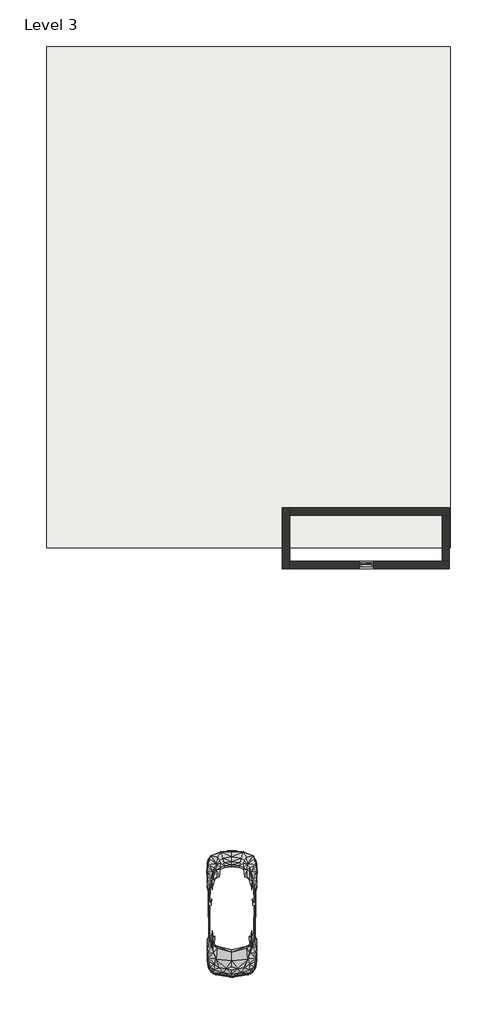
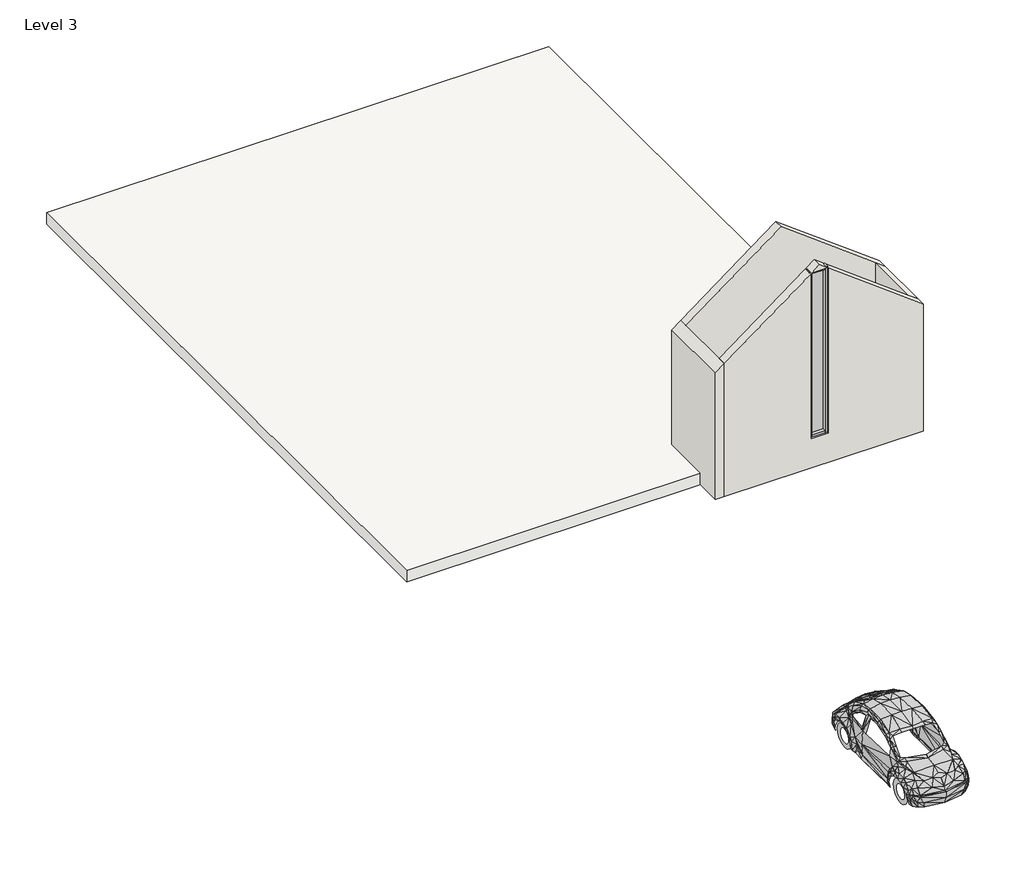
# One storey: 4 members, 4 walls, 1 plate, 1 proxy, 1 roof.
"""IFC4 building model written with IfcOpenShell, lengths in millimetres."""

from ifc_helpers import new_model, si_unit, frame, origin, place, context, project, spatial, polyline, outline, extrude, faceted_brep, transform, mapped, element, save
from components import rpc_beetle_rpc_beetle_31f8b51e, member_ff9f2d30, member_ad6a65ad, system_panel_glazed_5fe90612

model = new_model("IFC4")

# Units and contexts
model_context = context("Model", 3, world=origin())
ifc_project = project(units=[si_unit("LENGTHUNIT", "METRE", prefix="MILLI")], contexts=[model_context])

# Site, building, storey
site = spatial("IfcSite", under=ifc_project)
building = spatial("IfcBuilding", under=site)
storey = spatial("IfcBuildingStorey", under=building, Name="Level 3", Elevation=6096.0)

# Proxy
placement = place(None, origin())
rpc_beetle_rpc_beetle_shape = rpc_beetle_rpc_beetle_31f8b51e(model_context)
element("IfcBuildingElementProxy", 1, Name="RPC Beetle : RPC Beetle", ObjectType="RPC Beetle : RPC Beetle", at=placement, inside=storey, context=model_context, shape_type="MappedRepresentation", body=[
    mapped(rpc_beetle_rpc_beetle_shape, transform((-17655.2886697, -22453.5511954, 6096.0), x_axis=(-1.0, 0.0, 0.0), y_axis=(0.0, -1.0, 0.0), z_axis=(0.0, 0.0, 1.0))),
])

# Members
member_shape = member_ff9f2d30(model_context)
element("IfcMember", 2, ObjectType="Rectangular Mullion : 2.5\" x 5\" rectangular", at=placement, inside=storey, context=model_context, shape_type="MappedRepresentation", body=[
    mapped(member_shape, transform((-13610.3386697, -12750.7511954, 6863.106036), x_axis=(0.0, 0.0, -1.0), y_axis=(0.0, -1.0, 0.0), z_axis=(-1.0, 0.0, 0.0))),
])
element("IfcMember", 3, ObjectType="Rectangular Mullion : 2.5\" x 5\" rectangular", at=placement, inside=storey, context=model_context, shape_type="MappedRepresentation", body=[
    mapped(member_shape, transform((-13280.1386697, -12750.7511954, 11278.5636215), x_axis=(0.0, 0.0, 1.0), y_axis=(0.0, -1.0, 0.0), z_axis=(1.0, 0.0, 0.0))),
])
member_2_shape = member_ad6a65ad(model_context)
element("IfcMember", 4, ObjectType="Rectangular Mullion : 2.5\" x 5\" rectangular", at=placement, inside=storey, context=model_context, shape_type="MappedRepresentation", body=[
    mapped(member_2_shape, transform((-13673.8386697, -12750.7511954, 11278.5636215), x_axis=(-1.0, 0.0, 0.0), y_axis=(0.0, -1.0, 0.0), z_axis=(0.0, 0.0, 1.0))),
])
element("IfcMember", 5, ObjectType="Rectangular Mullion : 2.5\" x 5\" rectangular", at=placement, inside=storey, context=model_context, shape_type="MappedRepresentation", body=[
    mapped(member_2_shape, transform((-13216.6386697, -12750.7511954, 6863.106036), x_axis=(1.0, 0.0, 0.0), y_axis=(0.0, -1.0, 0.0), z_axis=(0.0, 0.0, -1.0))),
])

# Plate
system_panel_glazed_shape = system_panel_glazed_5fe90612(model_context)
element("IfcPlate", 6, ObjectType="System Panel : Glazed", at=placement, inside=storey, context=model_context, shape_type="MappedRepresentation", body=[
    mapped(system_panel_glazed_shape, transform((-13445.2386697, -12750.7511954, 6926.606036), x_axis=(1.0, 0.0, 0.0), y_axis=(0.0, 1.0, 0.0), z_axis=(0.0, 0.0, 1.0))),
])

# Roof
element("IfcRoof", 7, ObjectType="Generic - 12\"", at=placement, inside=storey, context=model_context, shape_type="SweptSolid", body=[
    extrude(outline(polyline([(-23465.5386697, 3492.5488046), (-10816.3386697, 3492.5488046), (-10816.3386697, -12204.6511954), (-23465.5386697, -12204.6511954), (-23465.5386697, 3492.5488046)])), frame((0.0, 0.0, 6096.0), z_axis=(0.0, 0.0, 1.0), x_axis=(1.0, 0.0, 0.0)), (0.0, 0.0, 1.0), 304.8),
])

# Walls
element("IfcWall", 8, ObjectType="9\"", at=placement, inside=storey, context=model_context, shape_type="Brep", body=[
    faceted_brep([(-15845.5386697, -12865.0511954, 6096.0), (-15845.5386697, -12636.4511954, 6096.0), (-15845.5386697, -11191.8261954, 6096.0), (-15845.5386697, -10963.2261954, 6096.0), (-15845.5386697, -10963.2261954, 9631.8623433), (-15845.5386697, -11191.8261954, 9631.8623433), (-15845.5386697, -12636.4511954, 9631.8623433), (-15845.5386697, -12865.0511954, 9631.8623433), (-16074.1386697, -12865.0511954, 6096.0), (-16074.1386697, -12865.0511954, 9460.4123433), (-16074.1386697, -10963.2261954, 9460.4123433), (-16074.1386697, -10963.2261954, 6096.0)], [[[0, 1, 2, 3, 4, 5, 6, 7]], [[8, 9, 10, 11]], [[3, 2, 1, 0, 8, 11]], [[4, 3, 11, 10]], [[0, 7, 9, 8]], [[7, 6, 5, 4, 10, 9]]]),
])
element("IfcWall", 9, ObjectType="9\"", at=placement, inside=storey, context=model_context, shape_type="Brep", body=[
    faceted_brep([(-15845.5386697, -11191.8261954, 6096.0), (-11070.3386697, -11191.8261954, 6096.0), (-10841.7386697, -11191.8261954, 6096.0), (-10841.7386697, -11191.8261954, 9471.8166443), (-11070.3386697, -11191.8261954, 9643.2666443), (-13450.3358024, -11191.8261954, 11428.2644938), (-15845.5386697, -11191.8261954, 9631.8623433), (-15845.5386697, -10963.2261954, 6096.0), (-15845.5386697, -10963.2261954, 9631.8623433), (-13450.3358024, -10963.2261954, 11428.2644938), (-10841.7386697, -10963.2261954, 9471.8166443), (-10841.7386697, -10963.2261954, 6096.0)], [[[0, 1, 2, 3, 4, 5, 6]], [[7, 8, 9, 10, 11]], [[2, 1, 0, 7, 11]], [[0, 6, 8, 7]], [[3, 2, 11, 10]], [[6, 5, 9, 8]], [[5, 4, 3, 10, 9]]]),
])
element("IfcWall", 10, ObjectType="9\"", at=placement, inside=storey, context=model_context, shape_type="Brep", body=[
    faceted_brep([(-15845.5386697, -12865.0511954, 6096.0), (-10841.7386697, -12865.0511954, 6096.0), (-10841.7386697, -12865.0511954, 9471.8166443), (-13216.6386697, -12865.0511954, 11252.9916443), (-13216.6386697, -12865.0511954, 6863.106036), (-13673.8386697, -12865.0511954, 6863.106036), (-13673.8386697, -12865.0511954, 11260.6373433), (-15845.5386697, -12865.0511954, 9631.8623433), (-10841.7386697, -12636.4511954, 6096.0), (-11070.3386697, -12636.4511954, 6096.0), (-15845.5386697, -12636.4511954, 6096.0), (-15845.5386697, -12636.4511954, 9631.8623433), (-13673.8386697, -12636.4511954, 11260.6373433), (-13673.8386697, -12636.4511954, 6863.106036), (-13216.6386697, -12636.4511954, 6863.106036), (-13216.6386697, -12636.4511954, 11252.9916443), (-11070.3386697, -12636.4511954, 9643.2666443), (-10841.7386697, -12636.4511954, 9471.8166443)], [[[0, 1, 2, 3, 4, 5, 6, 7]], [[8, 9, 10, 11, 12, 13, 14, 15, 16, 17]], [[0, 7, 11, 10]], [[2, 1, 8, 17]], [[11, 7, 6, 12]], [[2, 17, 16, 15, 3]], [[5, 13, 12, 6]], [[14, 4, 3, 15]], [[13, 5, 4, 14]], [[1, 0, 10, 9, 8]]]),
    faceted_brep([(-13250.7346392, -12865.0511954, 11278.5636215), (-13450.3358024, -12865.0511954, 11428.2644938), (-13649.9369655, -12865.0511954, 11278.5636215), (-13649.9369655, -12636.4511954, 11278.5636215), (-13450.3358024, -12636.4511954, 11428.2644938), (-13250.7346392, -12636.4511954, 11278.5636215)], [[[0, 1, 2]], [[3, 4, 5]], [[1, 4, 3, 2]], [[4, 1, 0, 5]], [[0, 2, 3, 5]]]),
])
element("IfcWall", 11, ObjectType="9\"", at=placement, inside=storey, context=model_context, shape_type="SweptSolid", body=[
    extrude(outline(polyline([(9643.2666443, -11070.3386697), (6096.0, -11070.3386697), (6096.0, -10841.7386697), (9471.8166443, -10841.7386697), (9643.2666443, -11070.3386697)])), frame((0.0, -12636.4511954, 0.0), z_axis=(0.0, 1.0, 0.0), x_axis=(0.0, 0.0, 1.0)), (0.0, 0.0, 1.0), 1444.625),
])

save(model, "model.ifc")

# Revit data of these elements
# Type "RPC Beetle : RPC Beetle"
#   built-in parameter 1005198 = "{2, 15},{39, RPC-16-0U6E-L4EG-ENH1-J3KF-SVEL-0TX4-C0},{1, 0},{1, 0},{2, 36},{1, 8},{5, Color},{1, 0},{1, 0},{3, 0.8},{3, 0.8},{3, 0.8},{1, 8},{7, BBoxMin},{1, 0},{1, 0},{1, 0},{1, 0},{1, 0},{1, 8},{7, BBoxMax},{1, 0},{1, 0},{1, 0},{1, 0},{1, 0},{2, 11},{9, RPCTypeId},{1, 0},{1, 0},{39, RPC-16-0U6E-L4EG-ENH1-J3KF-SVEL-0TX4-C0},{1, 6},{14, RPCPlantHeight},{1, 0},{1, 0},{7, 4.91667},{2, 11},{20, AdvancedUIDefinition},{1, 0},{1, 0},{0, },{2, 11},{10, AssetLibID},{1, 0},{1, 0},{36, 4D3F6E72-3F99-4203-98E9-AF80B3C7A7A4},{2, 11},{10, BaseSchema},{1, 0},{1, 0},{9, RPCSchema},{2, 11},{12, ExchangeGUID},{1, 0},{1, 0},{0, },{1, 2},{6, Hidden},{1, 0},{1, 0},{1, 0},{2, 11},{12, LocalizedUID},{1, 0},{1, 0},{0, },{1, 4},{11, RPCCategory},{1, 0},{1, 0},{1, 0},{2, 11},{8, RPCImage},{1, 0},{1, 0},{0, },{1, 4},{13, SchemaVersion},{1, 0},{1, 0},{1, 4},{2, 11},{12, UIDefinition},{1, 0},{1, 0},{0, },{2, 11},{6, UIName},{1, 0},{1, 0},{39, RPC-16-0U6E-L4EG-ENH1-J3KF-SVEL-0TX4-C0},{2, 11},{11, VersionGUID},{1, 0},{1, 0},{9, RPCSchema},{2, 11},{9, assettype},{1, 0},{1, 0},{11, RPCGeometry},{2, 11},{11, description},{1, 0},{1, 0},{0, },{2, 11},{9, localname},{1, 0},{1, 0},{3, RPC},{2, 11},{9, localtype},{1, 0},{1, 0},{3, RPC},{1, 4},{8, revision},{1, 0},{1, 0},{1, 1},{2, 11},{9, thumbnail},{1, 0},{1, 0},{0, },{1, 4},{7, version},{1, 0},{1, 0},{1, 1},{2, 14},{6, Height},{1, 0},{1, 0},{7, 4.91667},{1, 2},{20, RPC_Cast Reflections},{1, 0},{1, 0},{1, 1},{1, 4},{16, RPC_Transparency},{1, 0},{1, 0},{2, 18},{1, 4},{11, RPC_Tinting},{1, 0},{1, 0},{2, 50},{1, 2},{15, RPC_Use Tinting},{1, 0},{1, 0},{1, 0},{1, 2},{17, RPC_License Plate},{1, 0},{1, 0},{1, 0},{2, 11},{25, RPC_License Plate Texture},{1, 0},{1, 0},{64, __RPC:/object data/textures/car/plate/textures/default/rgb/0/0/0},{2, 11},{27, RPC_i_License Plate Texture},{1, 0},{1, 0},{0, },{1, 2},{16, RPC_Custom Plate},{1, 0},{1, 0},{1, 0},{2, 11},{27, RPC_License Plate File Name},{1, 0},{1, 0},{0, },{2, 11},{7, keyword},{1, 0},{1, 0},{27, :Geometry:RPC:VW Beetle [4]},{2, 11},{8, category},{1, 0},{1, 0},{21, :Auto_Economy/Midsize},{21, assetlibrary_base.fbx},{1, 5},"
#   built-in parameter 1005195 = "RPC-16-0U6E-L4EG-ENH1-J3KF-SVEL-0TX4-C0"
#   Height = 0
# Type "Rectangular Mullion : 2.5\" x 5\" rectangular"
#   built-in parameter 1007304 = 0.416667 (stored number, unit not read)
#   built-in parameter 1007301 = 0.104167 (stored number, unit not read)
#   built-in parameter 1007300 = 0.104167 (stored number, unit not read)
# Type "System Panel : Glazed"
#   Construction Type Id = "GSP4R"
#   Analytic Construction = "1/8 in Pilkington single glazing"
#   Visual Light Transmittance = 0.9
#   Solar Heat Gain Coefficient = 0.86
#   Heat Transfer Coefficient (U) = 1.18115 BTU/(h·ft²·°F)
#   Define Thermal Properties by = 1
# Type "Generic - 12\""
#   Assembly Code = "B1020"
#   Layers, outside or top first: 1' - 0" no material (function 1)
# Type "9\""
#   Assembly Code = "B2010"
#   Layers, outside or top first: 0' - 9" no material (function 1)
# Element 1 (IfcBuildingElementProxy, "RPC Beetle : RPC Beetle")
#   Phase Created = New Construction
# Elements 2, 3, 4, 5 (IfcMember, "Rectangular Mullion : 2.5\" x 5\" rectangular")
#   Phase Created = New Construction
#   Materials on its faces: "Aluminum"
# Element 6 (IfcPlate, "System Panel : Glazed")
#   Phase Created = New Construction
#   Materials on its faces: "Glass"
# Element 7 (IfcRoof, "Generic - 12\"")
#   built-in parameter 1001705 = 21 (stored number, unit not read)
#   built-in parameter 1001710 = 33615
#   Phase Created = New Construction
#   Materials on its faces: "Default Roof"
# Elements 8, 9, 10, 11 (IfcWall, "9\"")
#   Top Offset = 0' - 0"
#   Base Offset = 0' - 0"
#   Unconnected Height = 10' - 0"
#   wall height = 10' - 0"
#   Phase Created = New Construction
#   Base Constraint = Level 3
#   Materials on its faces: "Default Wall"
# Materials
#   "Aluminum": class "Metal", colour RGB 247 247 247, transparency 0, Description = "Aluminum 6061", Cost = 0
#   "Glass": class "Glass", colour RGB 0 128 192, transparency 0.75, Description = "Soda Lime Glass", Cost = 0
#   "Default Roof": colour RGB 88 101 114, transparency 0, Cost = 0
#   "Default Wall": colour RGB 128 128 128, transparency 0, Cost = 0
